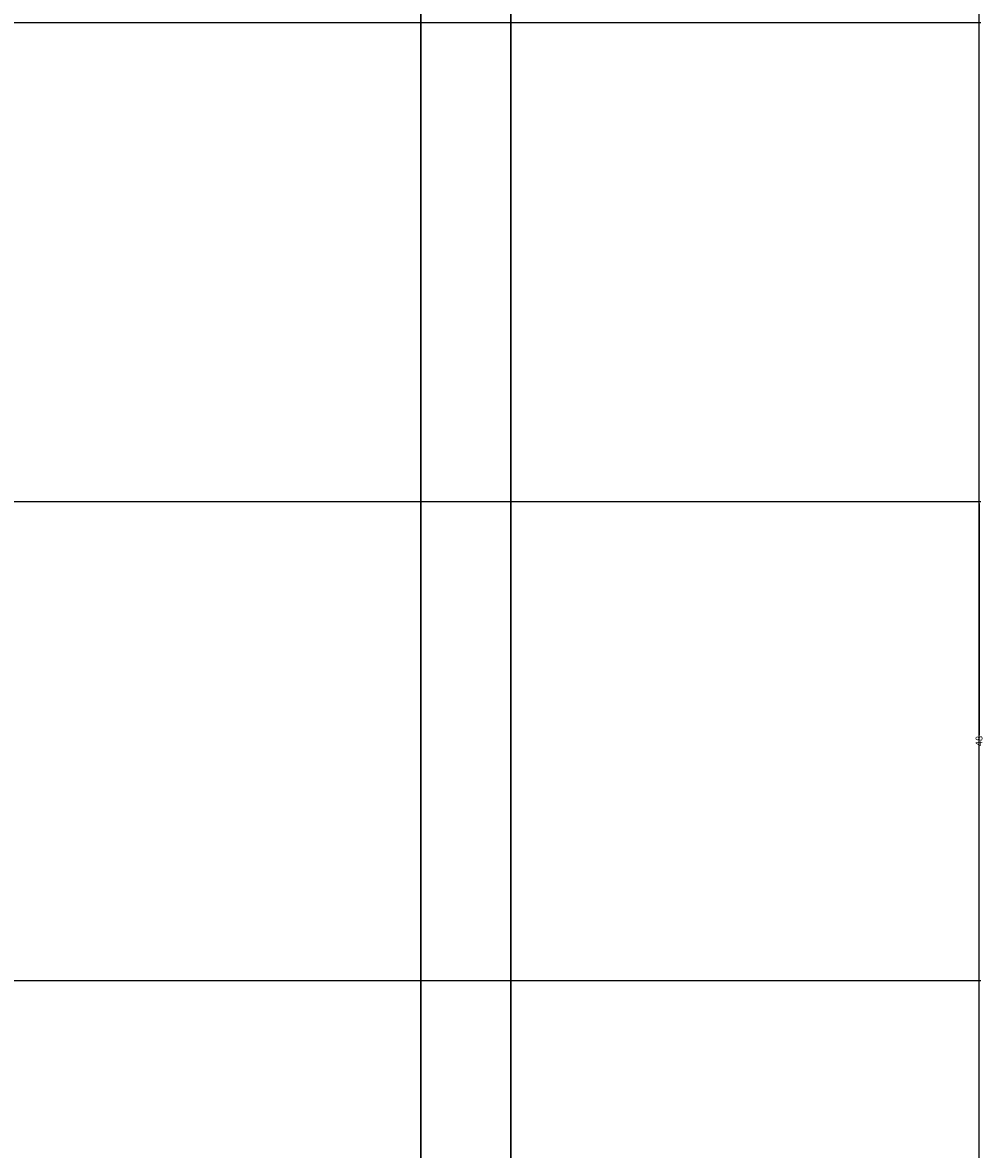
# Model space of a CAD drawing. Units: inches. Extents: x 867 to 1667, y -234 to 788.
# Tile 22 of 42: x 1571 to 1667, y -121 to -8. Entities that reach past the tile are written whole.
import ezdxf

# ---------------------------------------------------------------- set-up
doc = ezdxf.new("R2010")
doc.units = ezdxf.units.IN
doc.header["$MEASUREMENT"] = 0
doc.layers.add('A-ANNO-DIMS', color=2, linetype='Continuous', lineweight=18)
doc.layers.add('A-WALL-SITE', color=8, linetype='Continuous', lineweight=30)
doc.styles.get("Standard").update_dxf_attribs({"font": 'arial.ttf'})
doc.dimstyles.get("Standard").update_dxf_attribs({"dimtxt": 0.6875, "dimasz": 0.18, "dimexe": 0.18, "dimexo": 0.0625, "dimgap": 0.09, "dimtad": 0, "dimdec": 4, "dimzin": 0, "dimdsep": 46, "dimlunit": 4, "dimtxsty": 'Standard', "dimcen": 0.09, "dimadec": 0, "dimazin": 0, "dimtfac": 1, "dimtdec": 4, "dimtofl": 0, "dimtmove": 0, "dimatfit": 3, "dimfxl": 1, "dimtolj": 1, "dimtzin": 0, "dimarcsym": 0})

# ---------------------------------------------------------------- blocks, each defined once
blk = doc.blocks.new('*D18')
at = {"layer": 'A-ANNO-DIMS', "color": 0, "lineweight": -2, "transparency": 16777216}
for p, q in [((1619.95, 740.62), (1667.02, 740.62)), ((1666.84, 740.44), (1666.84, 277.95)), ((1666.84, -186.23), (1666.84, 276.25)), ((1619.95, -186.41), (1667.02, -186.41))]:
    blk.add_line(p, q, dxfattribs=at)
at = {"layer": 'A-ANNO-DIMS', "color": 0, "transparency": 16777216}
for points in [[(1666.81, 740.44), (1666.87, 740.44), (1666.84, 740.62)], [(1666.81, -186.23), (1666.87, -186.23), (1666.84, -186.41)]]:
    blk.add_solid(points, dxfattribs=at)
at = {"layer": 'Defpoints', "color": 0, "transparency": 16777216}
for p in [(1619.89, 740.62), (1666.84, 740.62), (1619.89, -186.41)]:
    blk.add_point(p, dxfattribs=at)
at = {"layer": 'A-ANNO-DIMS', "color": 0, "transparency": 16777216, "insert": (1666.84, 277.1), "char_height": 0.688, "attachment_point": 5, "rotation": 90}
blk.add_mtext('\\A1;927', dxfattribs=at)
blk = doc.blocks.new('*D51')
at = {"layer": 'A-ANNO-DIMS', "color": 0, "lineweight": -2, "transparency": 16777216}
for p, q in [((1391.95, -55.91), (1667.02, -55.91)), ((1666.84, -56.09), (1666.84, -79.31)), ((1666.84, -103.73), (1666.84, -80.51)), ((1391.95, -103.91), (1667.02, -103.91))]:
    blk.add_line(p, q, dxfattribs=at)
at = {"layer": 'A-ANNO-DIMS', "color": 0, "transparency": 16777216}
for points in [[(1666.81, -56.09), (1666.87, -56.09), (1666.84, -55.91)], [(1666.81, -103.73), (1666.87, -103.73), (1666.84, -103.91)]]:
    blk.add_solid(points, dxfattribs=at)
at = {"layer": 'Defpoints', "color": 0, "transparency": 16777216}
for p in [(1391.89, -55.91), (1391.89, -103.91), (1666.84, -103.91)]:
    blk.add_point(p, dxfattribs=at)
at = {"layer": 'A-ANNO-DIMS', "color": 0, "transparency": 16777216, "insert": (1666.84, -79.91), "char_height": 0.688, "attachment_point": 5, "rotation": 90}
blk.add_mtext('\\A1;48', dxfattribs=at)
blk = doc.blocks.new('*D59')
at = {"layer": 'A-ANNO-DIMS', "color": 0, "lineweight": -2, "transparency": 16777216}
for p, q in [((1559.95, 24.65), (1667.02, 24.65)), ((1666.84, 24.47), (1666.84, 9.9)), ((1666.84, -7.7), (1666.84, 6.87)), ((1559.95, -7.88), (1667.02, -7.88))]:
    blk.add_line(p, q, dxfattribs=at)
at = {"layer": 'A-ANNO-DIMS', "color": 0, "transparency": 16777216}
for points in [[(1666.81, 24.47), (1666.87, 24.47), (1666.84, 24.65)], [(1666.81, -7.7), (1666.87, -7.7), (1666.84, -7.88)]]:
    blk.add_solid(points, dxfattribs=at)
at = {"layer": 'Defpoints', "color": 0, "transparency": 16777216}
for p in [(1559.89, 24.65), (1666.84, 24.65), (1559.89, -7.88)]:
    blk.add_point(p, dxfattribs=at)
at = {"layer": 'A-ANNO-DIMS', "color": 0, "transparency": 16777216, "insert": (1666.84, 8.38), "char_height": 0.688, "attachment_point": 5, "rotation": 90}
blk.add_mtext('\\A1;32.534', dxfattribs=at)

msp = doc.modelspace()

# ---------------------------------------------------------------- linework, layer by layer
at = {"layer": 'A-WALL-SITE'}
for p, q in [((1610.8866, 740.617), (1610.8866, -186.4081)), ((1619.8866, 740.617), (1619.8866, -186.4081))]:
    msp.add_line(p, q, dxfattribs=at)

# ---------------------------------------------------------------- dimensions: what is measured, and where the dimension line sits
at = {"layer": 'A-ANNO-DIMS'}
for base, p1, p2, override, picture, middle in [((1666.8366, 740.617), (1619.8866, -186.4081), (1619.8866, 740.617), {"dimdec": 0, "dimlfac": 1, "dimrnd": 0, "dimzin": 0, "dimdsep": 46, "dimlunit": 2}, '*D18', (1666.8366, 277.1045)), ((1666.8366, 24.6511), (1559.8866, -7.883), (1559.8866, 24.6511), {"dimdec": 3, "dimlfac": 1, "dimrnd": 0, "dimzin": 0, "dimdsep": 46, "dimlunit": 2}, '*D59', (1666.8366, 8.3841)), ((1666.8366, -103.9081), (1391.8866, -55.9081), (1391.8866, -103.9081), {"dimdec": 0, "dimlfac": 1, "dimrnd": 0, "dimzin": 0, "dimdsep": 46, "dimlunit": 2}, '*D51', (1666.8366, -79.9081))]:
    dim = msp.add_linear_dim(base=base, p1=p1, p2=p2, angle=90, dimstyle='Standard', override=override, dxfattribs=at)
    dim.commit()
    dim.dimension.update_dxf_attribs({"geometry": picture, "text_midpoint": middle})

doc.saveas('drawing.dxf')
